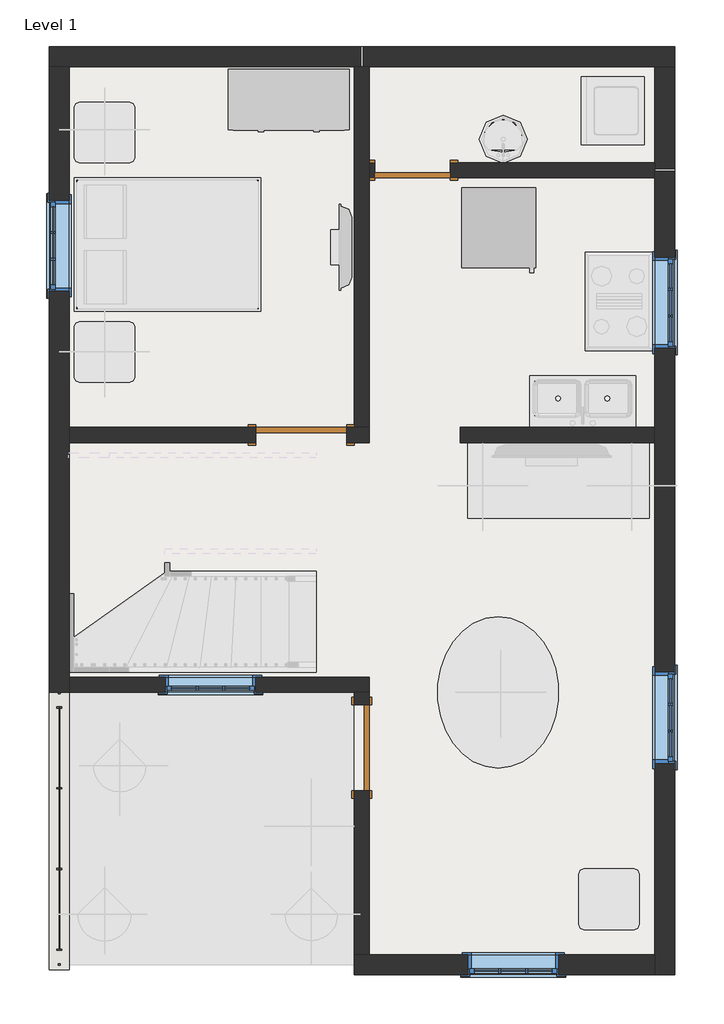
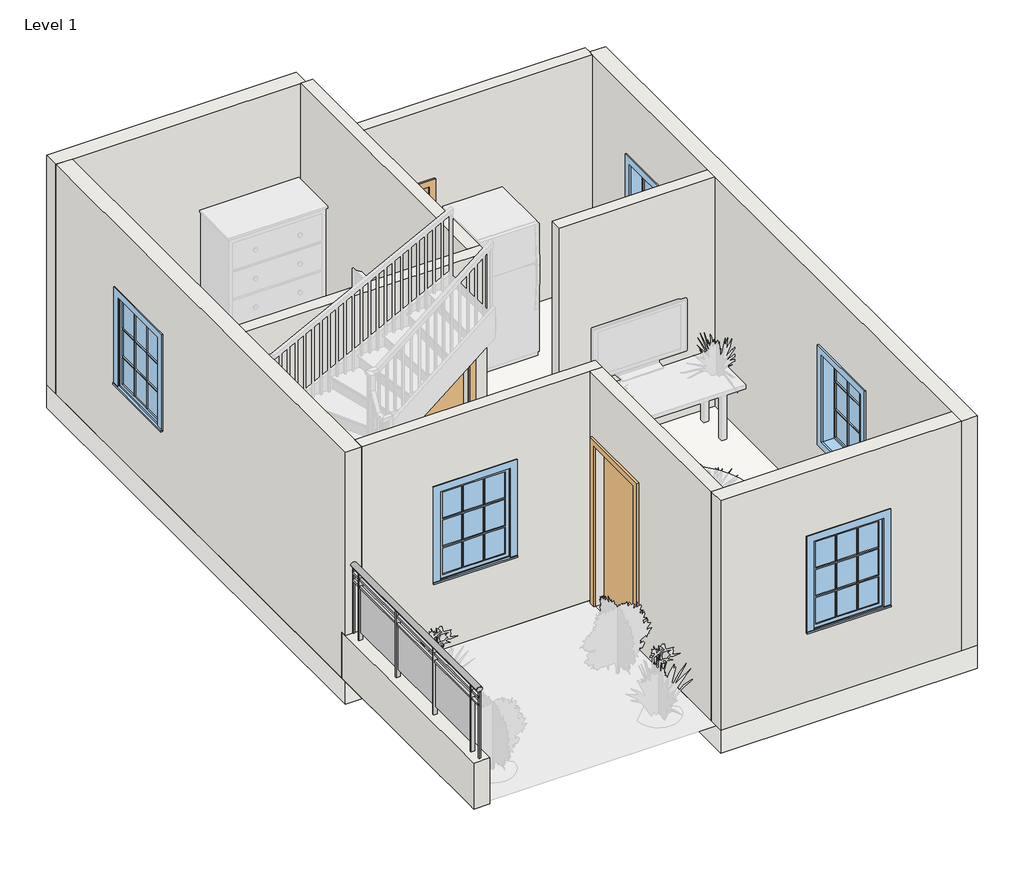
# One storey, part 1 of 3: 13 walls, 5 windows, 3 doors, 1 railing, 1 slab.
"""IFC4 building model written with IfcOpenShell, lengths in millimetres."""

from ifc_helpers import new_model, si_unit, point, frame, origin, origin_with_axes, place, context, project, spatial, polyline, ellipse_curve, trimmed, outline, extrude, faceted_brep, transform, mapped, element, save
from ifc_brep_helpers import plane_surface, extruded_surface, advanced_brep
from components import door_059fdd7e, door_b6e9fca3, door_16372e1c, window_29c06734, window_5c190c7e

model = new_model("IFC4")

# Units and contexts
model_context = context("Model", 3, world=origin())
ifc_project = project(units=[si_unit("LENGTHUNIT", "METRE", prefix="MILLI")], contexts=[model_context])

# Site, building, storey
site = spatial("IfcSite", under=ifc_project)
building = spatial("IfcBuilding", under=site)
storey = spatial("IfcBuildingStorey", under=building, Name="Level 1", Elevation=0.0)

# Doors
placement = place(None, origin())
door_shape = door_059fdd7e(model_context)
element("IfcDoor", 1, ObjectType="Single-Flush : 30\" x 80\"", at=placement, inside=storey, context=model_context, shape_type="MappedRepresentation", body=[
    mapped(door_shape, transform((-13127.2170266, 11870.4465295, 0.0), x_axis=(-1.0, 0.0, 0.0), y_axis=(0.0, -1.0, 0.0), z_axis=(0.0, 0.0, 1.0))),
])
door_2_shape = door_b6e9fca3(model_context)
element("IfcDoor", 2, ObjectType="Single-Flush : 34\" x 84\"", at=placement, inside=storey, context=model_context, shape_type="MappedRepresentation", body=[
    mapped(door_2_shape, transform((-13635.2170266, 6053.8465295, 0.0), x_axis=(0.0, -1.0, 0.0), y_axis=(1.0, 0.0, 0.0), z_axis=(0.0, 0.0, 1.0))),
])
door_3_shape = door_16372e1c(model_context)
element("IfcDoor", 3, ObjectType="Single-Flush : 36\" x 84\"", at=placement, inside=storey, context=model_context, shape_type="MappedRepresentation", body=[
    mapped(door_3_shape, transform((-14244.8170266, 9203.4465295, 0.0), x_axis=(1.0, 0.0, 0.0), y_axis=(0.0, 1.0, 0.0), z_axis=(0.0, 0.0, 1.0))),
])

# Railing
element("IfcRailing", 4, ObjectType="Glass Panel - Bottom Fill", at=placement, inside=storey, context=model_context, shape_type="SolidModel", body=[
    advanced_brep(
    [(-16645.1170266, 6612.6465295, 1524.0), (-16721.3170266, 6612.6465295, 1524.0), (-16645.1170266, 3869.4465295, 1524.0), (-16721.3170266, 3869.4465295, 1524.0)],
    [
        (0, 1, ellipse_curve(frame((-16683.2170266, 6612.6465295, 1524.0), z_axis=(0.0, 1.0, 0.0), x_axis=(-1.0, 0.0, 0.0)), 38.1, 28.575)),
        (1, 0, ellipse_curve(frame((-16683.2170266, 6612.6465295, 1524.0), z_axis=(0.0, 1.0, 0.0), x_axis=(-1.0, 0.0, 0.0)), 38.1, 28.575)),
        (2, 3, ellipse_curve(frame((-16683.2170266, 3869.4465295, 1524.0), z_axis=(0.0, -1.0, 0.0), x_axis=(-1.0, 0.0, 0.0)), 38.1, 28.575)),
        (3, 2, ellipse_curve(frame((-16683.2170266, 3869.4465295, 1524.0), z_axis=(0.0, -1.0, 0.0), x_axis=(-1.0, 0.0, 0.0)), 38.1, 28.575)),
        (0, 2),
        (3, 1),
    ],
    [
        plane_surface(frame((-16683.2170266, 6612.6465295, 1524.0), z_axis=(0.0, 1.0, 0.0), x_axis=(0.0, 0.0, -1.0))),
        plane_surface(frame((-16683.2170266, 3869.4465295, 1524.0), z_axis=(0.0, -1.0, 0.0), x_axis=(0.0, 0.0, -1.0))),
        extruded_surface(trimmed(ellipse_curve(frame((-16683.2170266, 3869.4465295, 1524.0), z_axis=(0.0, 1.0, 0.0), x_axis=(-1.0, 0.0, 0.0)), 38.1, 28.575), [point((-16645.1170266, 3869.4465295, 1524.0))], [point((-16721.3170266, 3869.4465295, 1524.0))], True, "CARTESIAN"), (0.0, 2743.2, 0.0), 2743.2),
        extruded_surface(trimmed(ellipse_curve(frame((-16683.2170266, 3869.4465295, 1524.0), z_axis=(0.0, 1.0, 0.0), x_axis=(-1.0, 0.0, 0.0)), 38.1, 28.575), [point((-16721.3170266, 3869.4465295, 1524.0))], [point((-16645.1170266, 3869.4465295, 1524.0))], True, "CARTESIAN"), (0.0, 2743.2, 0.0), 2743.2),
    ],
    [
        (0, [[1, 2]]),
        (1, [[3, 4]]),
        (2, [[-1, 5, -4, 6]]),
        (3, [[-2, -6, -3, -5]]),
    ],
),
    extrude(outline(polyline([(-16695.9170266, 6612.6465295), (-16670.5170266, 6612.6465295), (-16670.5170266, 3869.4465295), (-16695.9170266, 3869.4465295), (-16695.9170266, 6612.6465295)])), frame((0.0, 0.0, 1409.7), z_axis=(0.0, 0.0, 1.0), x_axis=(1.0, 0.0, 0.0)), (0.0, 0.0, 1.0), 25.4),
    extrude(outline(polyline([(-16695.9170266, 6612.6465295), (-16670.5170266, 6612.6465295), (-16670.5170266, 3869.4465295), (-16695.9170266, 3869.4465295), (-16695.9170266, 6612.6465295)])), frame((0.0, 0.0, 1308.1), z_axis=(0.0, 0.0, 1.0), x_axis=(1.0, 0.0, 0.0)), (0.0, 0.0, 1.0), 25.4),
    extrude(outline(polyline([(-16708.6170266, 4028.1965295), (-16657.8170266, 4028.1965295), (-16657.8170266, 4015.4965295), (-16708.6170266, 4015.4965295), (-16708.6170266, 4028.1965295)])), frame((0.0, 0.0, 609.6), z_axis=(0.0, 0.0, 1.0), x_axis=(1.0, 0.0, 0.0)), (0.0, 0.0, 1.0), 885.6788223),
    extrude(outline(polyline([(-16676.6818696, 4834.6465295), (-16676.6818696, 4021.8465295), (-16683.0318696, 4021.8465295), (-16683.0318696, 4834.6465295), (-16676.6818696, 4834.6465295)])), frame((0.0, 0.0, 711.2), z_axis=(0.0, 0.0, 1.0), x_axis=(1.0, 0.0, 0.0)), (0.0, 0.0, 1.0), 596.9),
    extrude(outline(polyline([(-16708.6170266, 4840.9965295), (-16657.8170266, 4840.9965295), (-16657.8170266, 4828.2965295), (-16708.6170266, 4828.2965295), (-16708.6170266, 4840.9965295)])), frame((0.0, 0.0, 609.6), z_axis=(0.0, 0.0, 1.0), x_axis=(1.0, 0.0, 0.0)), (0.0, 0.0, 1.0), 885.6788223),
    extrude(outline(polyline([(-16676.6818696, 5647.4465295), (-16676.6818696, 4834.6465295), (-16683.0318696, 4834.6465295), (-16683.0318696, 5647.4465295), (-16676.6818696, 5647.4465295)])), frame((0.0, 0.0, 711.2), z_axis=(0.0, 0.0, 1.0), x_axis=(1.0, 0.0, 0.0)), (0.0, 0.0, 1.0), 596.9),
    extrude(outline(polyline([(-16708.6170266, 5653.7965295), (-16657.8170266, 5653.7965295), (-16657.8170266, 5641.0965295), (-16708.6170266, 5641.0965295), (-16708.6170266, 5653.7965295)])), frame((0.0, 0.0, 609.6), z_axis=(0.0, 0.0, 1.0), x_axis=(1.0, 0.0, 0.0)), (0.0, 0.0, 1.0), 885.6788223),
    extrude(outline(polyline([(-16676.6818696, 6460.2465295), (-16676.6818696, 5647.4465295), (-16683.0318696, 5647.4465295), (-16683.0318696, 6460.2465295), (-16676.6818696, 6460.2465295)])), frame((0.0, 0.0, 711.2), z_axis=(0.0, 0.0, 1.0), x_axis=(1.0, 0.0, 0.0)), (0.0, 0.0, 1.0), 596.9),
    extrude(outline(polyline([(-16708.6170266, 6466.5965295), (-16657.8170266, 6466.5965295), (-16657.8170266, 6453.8965295), (-16708.6170266, 6453.8965295), (-16708.6170266, 6466.5965295)])), frame((0.0, 0.0, 609.6), z_axis=(0.0, 0.0, 1.0), x_axis=(1.0, 0.0, 0.0)), (0.0, 0.0, 1.0), 885.6788223),
    extrude(outline(polyline([(-16692.7420266, 3882.1465295), (-16673.6920266, 3882.1465295), (-16673.6920266, 3863.0965295), (-16692.7420266, 3863.0965295), (-16692.7420266, 3882.1465295)])), frame((0.0, 0.0, 609.6), z_axis=(0.0, 0.0, 1.0), x_axis=(1.0, 0.0, 0.0)), (0.0, 0.0, 1.0), 885.6788223),
    extrude(outline(polyline([(-16692.7420266, 6618.9965295), (-16673.6920266, 6618.9965295), (-16673.6920266, 6599.9465295), (-16692.7420266, 6599.9465295), (-16692.7420266, 6618.9965295)])), frame((0.0, 0.0, 609.6), z_axis=(0.0, 0.0, 1.0), x_axis=(1.0, 0.0, 0.0)), (0.0, 0.0, 1.0), 885.6788223),
])

# Slab
element("IfcSlab", 5, ObjectType="Generic - 12\"", at=placement, inside=storey, context=model_context, shape_type="SweptSolid", body=[
    extrude(outline(polyline([(-10485.6170266, 13115.0465295), (-10485.6170266, 3767.8465295), (-13711.4170266, 3767.8465295), (-13711.4170266, 6612.6465295), (-16784.8170266, 6612.6465295), (-16784.8170266, 13115.0465295), (-10485.6170266, 13115.0465295)])), frame((0.0, 0.0, -304.8), z_axis=(0.0, 0.0, 1.0), x_axis=(1.0, 0.0, 0.0)), (0.0, 0.0, 1.0), 304.8),
])

# Walls
element("IfcWall", 6, ObjectType="Generic - 8\"", at=placement, inside=storey, context=model_context, shape_type="Brep", body=[
    faceted_brep([(-13711.4170266, 12911.8465295, 0.0), (-13711.4170266, 9279.6465295, 0.0), (-13711.4170266, 9279.6465295, 3048.0), (-13711.4170266, 12911.8465295, 3048.0), (-13559.0170266, 12911.8465295, 0.0), (-13559.0170266, 12911.8465295, 3048.0), (-13559.0170266, 11946.6465295, 3048.0), (-13559.0170266, 11794.2465295, 3048.0), (-13559.0170266, 9279.6465295, 3048.0), (-13559.0170266, 9279.6465295, 0.0), (-13559.0170266, 11794.2465295, 0.0), (-13559.0170266, 11946.6465295, 0.0), (-13622.5170266, 12911.8465295, 0.0)], [[[0, 1, 2, 3]], [[4, 5, 6, 7, 8, 9, 10, 11]], [[1, 0, 12, 4, 11, 10, 9]], [[3, 2, 8, 7, 6, 5]], [[0, 3, 5, 4, 12]], [[2, 1, 9, 8]]]),
])
element("IfcWall", 7, ObjectType="Generic - 8\"", at=placement, inside=storey, context=model_context, shape_type="SweptSolid", body=[
    extrude(outline(polyline([(-12644.6170266, 9279.6465295), (-10688.8170266, 9279.6465295), (-10688.8170266, 9127.2465295), (-12644.6170266, 9127.2465295), (-12644.6170266, 9279.6465295)])), origin_with_axes(), (0.0, 0.0, 1.0), 3048.0),
])
element("IfcWall", 8, ObjectType="Generic - 8\"", at=placement, inside=storey, context=model_context, shape_type="Brep", body=[
    faceted_brep([(-13559.0170266, 11794.2465295, 0.0), (-13508.2170266, 11794.2465295, 0.0), (-13508.2170266, 11794.2465295, 2032.0), (-12746.2170266, 11794.2465295, 2032.0), (-12746.2170266, 11794.2465295, 0.0), (-10688.8170266, 11794.2465295, 0.0), (-10688.8170266, 11794.2465295, 3048.0), (-13559.0170266, 11794.2465295, 3048.0), (-13508.2170266, 11946.6465295, 2032.0), (-13508.2170266, 11946.6465295, 0.0), (-13559.0170266, 11946.6465295, 0.0), (-13559.0170266, 11946.6465295, 3048.0), (-10688.8170266, 11946.6465295, 3048.0), (-10688.8170266, 11946.6465295, 0.0), (-12746.2170266, 11946.6465295, 0.0), (-12746.2170266, 11946.6465295, 2032.0), (-10688.8170266, 11857.7465295, 0.0), (-10688.8170266, 11857.7465295, 3048.0)], [[[0, 1, 2, 3, 4, 5, 6, 7]], [[8, 9, 10, 11, 12, 13, 14, 15]], [[14, 13, 16, 5, 4]], [[10, 9, 1, 0]], [[7, 6, 17, 12, 11]], [[6, 5, 16, 13, 12, 17]], [[0, 7, 11, 10]], [[2, 1, 9, 8]], [[3, 2, 8, 15]], [[4, 3, 15, 14]]]),
])
element("IfcWall", 9, ObjectType="Generic - 8\"", at=placement, inside=storey, context=model_context, shape_type="Brep", body=[
    faceted_brep([(-16581.6170266, 6612.6465295, 3048.0), (-16581.6170266, 6612.6465295, 609.6), (-16581.6170266, 6612.6465295, 0.0), (-13711.4170266, 6612.6465295, 0.0), (-13559.0170266, 6612.6465295, 0.0), (-13559.0170266, 6612.6465295, 3048.0), (-13711.4170266, 6612.6465295, 3048.0), (-15616.4170266, 6612.6465295, 2133.6), (-14702.0170266, 6612.6465295, 2133.6), (-14702.0170266, 6612.6465295, 914.4), (-15616.4170266, 6612.6465295, 914.4), (-16581.6170266, 6765.0465295, 0.0), (-16581.6170266, 6765.0465295, 3048.0), (-13559.0170266, 6765.0465295, 3048.0), (-13559.0170266, 6765.0465295, 0.0), (-15616.4170266, 6765.0465295, 2133.6), (-15616.4170266, 6765.0465295, 914.4), (-14702.0170266, 6765.0465295, 914.4), (-14702.0170266, 6765.0465295, 2133.6), (-16581.6170266, 6688.8465295, 0.0)], [[[0, 1, 2, 3, 4, 5, 6], [7, 8, 9, 10]], [[11, 12, 13, 14], [15, 16, 17, 18]], [[4, 3, 2, 19, 11, 14]], [[0, 6, 5, 13, 12]], [[5, 4, 14, 13]], [[0, 12, 11, 19, 2, 1]], [[16, 15, 7, 10]], [[17, 16, 10, 9]], [[18, 17, 9, 8]], [[15, 18, 8, 7]]]),
])
element("IfcWall", 10, ObjectType="Generic - 8\"", at=placement, inside=storey, context=model_context, shape_type="SweptSolid", body=[
    extrude(outline(polyline([(5622.0465295, 2133.6), (5622.0465295, 0.0), (3971.0465295, 0.0), (3971.0465295, 3048.0), (6612.6465295, 3048.0), (6612.6465295, 0.0), (6485.6465295, 0.0), (6485.6465295, 2133.6), (5622.0465295, 2133.6)])), frame((-13711.4170266, 0.0, 0.0), z_axis=(1.0, 0.0, 0.0), x_axis=(0.0, 1.0, 0.0)), (0.0, 0.0, 1.0), 152.4),
])
element("IfcWall", 11, ObjectType="Generic - 8\"", at=placement, inside=storey, context=model_context, shape_type="Brep", body=[
    faceted_brep([(-13559.0170266, 9279.6465295, 0.0), (-13711.4170266, 9279.6465295, 0.0), (-13787.6170266, 9279.6465295, 0.0), (-13787.6170266, 9279.6465295, 2133.6), (-14702.0170266, 9279.6465295, 2133.6), (-14702.0170266, 9279.6465295, 0.0), (-16581.6170266, 9279.6465295, 0.0), (-16581.6170266, 9279.6465295, 3048.0), (-13711.4170266, 9279.6465295, 3048.0), (-13559.0170266, 9279.6465295, 3048.0), (-13787.6170266, 9127.2465295, 2133.6), (-13787.6170266, 9127.2465295, 0.0), (-13559.0170266, 9127.2465295, 0.0), (-13559.0170266, 9127.2465295, 3048.0), (-16581.6170266, 9127.2465295, 3048.0), (-16581.6170266, 9127.2465295, 0.0), (-14702.0170266, 9127.2465295, 0.0), (-14702.0170266, 9127.2465295, 2133.6)], [[[0, 1, 2, 3, 4, 5, 6, 7, 8, 9]], [[10, 11, 12, 13, 14, 15, 16, 17]], [[16, 15, 6, 5]], [[12, 11, 2, 1, 0]], [[9, 8, 7, 14, 13]], [[7, 6, 15, 14]], [[5, 4, 17, 16]], [[4, 3, 10, 17]], [[3, 2, 11, 10]], [[0, 9, 13, 12]]]),
])
element("IfcWall", 12, ObjectType="Generic - 8\" 2", at=placement, inside=storey, context=model_context, shape_type="Brep", body=[
    faceted_brep([(-16784.8170266, 12911.8465295, 0.0), (-16581.6170266, 12911.8465295, 0.0), (-13647.9170266, 12911.8465295, 0.0), (-13647.9170266, 12911.8465295, 3048.0), (-16581.6170266, 12911.8465295, 3048.0), (-16784.8170266, 12911.8465295, 3048.0), (-16784.8170266, 13115.0465295, 0.0), (-16784.8170266, 13115.0465295, 3048.0), (-13647.9170266, 13115.0465295, 3048.0), (-13647.9170266, 13115.0465295, 0.0)], [[[0, 1, 2, 3, 4, 5]], [[6, 7, 8, 9]], [[2, 1, 0, 6, 9]], [[3, 2, 9, 8]], [[5, 4, 3, 8, 7]], [[0, 5, 7, 6]]]),
])
element("IfcWall", 13, ObjectType="Generic - 8\" 2", at=placement, inside=storey, context=model_context, shape_type="SweptSolid", body=[
    extrude(outline(polyline([(-10688.8170266, 11883.1465295), (-10688.8170266, 12911.8465295), (-10485.6170266, 12911.8465295), (-10485.6170266, 11883.1465295), (-10688.8170266, 11883.1465295)])), origin_with_axes(), (0.0, 0.0, 1.0), 1524.0),
])
element("IfcWall", 14, ObjectType="Generic - 8\" 2", at=placement, inside=storey, context=model_context, shape_type="Brep", body=[
    faceted_brep([(-10688.8170266, 3971.0465295, 0.0), (-13559.0170266, 3971.0465295, 0.0), (-13711.4170266, 3971.0465295, 0.0), (-13711.4170266, 3971.0465295, 3048.0), (-13559.0170266, 3971.0465295, 3048.0), (-10688.8170266, 3971.0465295, 3048.0), (-12568.4170266, 3971.0465295, 2133.6), (-12568.4170266, 3971.0465295, 914.4), (-11654.0170266, 3971.0465295, 914.4), (-11654.0170266, 3971.0465295, 2133.6), (-10688.8170266, 3767.8465295, 0.0), (-10688.8170266, 3767.8465295, 3048.0), (-13711.4170266, 3767.8465295, 3048.0), (-13711.4170266, 3767.8465295, 0.0), (-12568.4170266, 3767.8465295, 2133.6), (-11654.0170266, 3767.8465295, 2133.6), (-11654.0170266, 3767.8465295, 914.4), (-12568.4170266, 3767.8465295, 914.4)], [[[0, 1, 2, 3, 4, 5], [6, 7, 8, 9]], [[10, 11, 12, 13], [14, 15, 16, 17]], [[2, 1, 0, 10, 13]], [[5, 4, 3, 12, 11]], [[0, 5, 11, 10]], [[3, 2, 13, 12]], [[7, 6, 14, 17]], [[8, 7, 17, 16]], [[9, 8, 16, 15]], [[6, 9, 15, 14]]]),
])
element("IfcWall", 15, ObjectType="Generic - 8\" 2", at=placement, inside=storey, context=model_context, shape_type="Brep", body=[
    faceted_brep([(-13622.5170266, 12911.8465295, 0.0), (-13559.0170266, 12911.8465295, 0.0), (-10688.8170266, 12911.8465295, 0.0), (-10485.6170266, 12911.8465295, 0.0), (-10485.6170266, 12911.8465295, 1524.0), (-10688.8170266, 12911.8465295, 1524.0), (-13622.5170266, 12911.8465295, 1524.0), (-13622.5170266, 13115.0465295, 0.0), (-13622.5170266, 13115.0465295, 1524.0), (-10485.6170266, 13115.0465295, 1524.0), (-10485.6170266, 13115.0465295, 0.0)], [[[0, 1, 2, 3, 4, 5, 6]], [[7, 8, 9, 10]], [[3, 2, 1, 0, 7, 10]], [[6, 5, 4, 9, 8]], [[0, 6, 8, 7]], [[4, 3, 10, 9]]]),
])
element("IfcWall", 16, ObjectType="Generic - 8\" 2", at=placement, inside=storey, context=model_context, shape_type="Brep", body=[
    faceted_brep([(-10688.8170266, 11857.7465295, 0.0), (-10688.8170266, 11794.2465295, 0.0), (-10688.8170266, 9279.6465295, 0.0), (-10688.8170266, 9127.2465295, 0.0), (-10688.8170266, 3971.0465295, 0.0), (-10688.8170266, 3767.8465295, 0.0), (-10688.8170266, 3767.8465295, 3048.0), (-10688.8170266, 3971.0465295, 3048.0), (-10688.8170266, 9127.2465295, 3048.0), (-10688.8170266, 9279.6465295, 3048.0), (-10688.8170266, 11794.2465295, 3048.0), (-10688.8170266, 11857.7465295, 3048.0), (-10688.8170266, 10079.7465295, 2133.6), (-10688.8170266, 10079.7465295, 914.4), (-10688.8170266, 10994.1465295, 914.4), (-10688.8170266, 10994.1465295, 2133.6), (-10688.8170266, 5901.4465295, 2133.6), (-10688.8170266, 5901.4465295, 914.4), (-10688.8170266, 6815.8465295, 914.4), (-10688.8170266, 6815.8465295, 2133.6), (-10485.6170266, 11857.7465295, 0.0), (-10485.6170266, 11857.7465295, 3048.0), (-10485.6170266, 3767.8465295, 3048.0), (-10485.6170266, 3767.8465295, 0.0), (-10485.6170266, 10079.7465295, 2133.6), (-10485.6170266, 10994.1465295, 2133.6), (-10485.6170266, 10994.1465295, 914.4), (-10485.6170266, 10079.7465295, 914.4), (-10485.6170266, 5901.4465295, 2133.6), (-10485.6170266, 6815.8465295, 2133.6), (-10485.6170266, 6815.8465295, 914.4), (-10485.6170266, 5901.4465295, 914.4)], [[[0, 1, 2, 3, 4, 5, 6, 7, 8, 9, 10, 11], [12, 13, 14, 15], [16, 17, 18, 19]], [[20, 21, 22, 23], [24, 25, 26, 27], [28, 29, 30, 31]], [[5, 4, 3, 2, 1, 0, 20, 23]], [[11, 10, 9, 8, 7, 6, 22, 21]], [[0, 11, 21, 20]], [[6, 5, 23, 22]], [[13, 12, 24, 27]], [[14, 13, 27, 26]], [[15, 14, 26, 25]], [[12, 15, 25, 24]], [[17, 16, 28, 31]], [[18, 17, 31, 30]], [[19, 18, 30, 29]], [[16, 19, 29, 28]]]),
])
element("IfcWall", 17, ObjectType="Generic - 8\" 2", at=placement, inside=storey, context=model_context, shape_type="Brep", body=[
    faceted_brep([(-16581.6170266, 6688.8465295, 0.0), (-16581.6170266, 6765.0465295, 0.0), (-16581.6170266, 9127.2465295, 0.0), (-16581.6170266, 9279.6465295, 0.0), (-16581.6170266, 12911.8465295, 0.0), (-16581.6170266, 12911.8465295, 3048.0), (-16581.6170266, 9279.6465295, 3048.0), (-16581.6170266, 9127.2465295, 3048.0), (-16581.6170266, 6765.0465295, 3048.0), (-16581.6170266, 6612.6465295, 3048.0), (-16581.6170266, 6612.6465295, 609.6), (-16581.6170266, 6688.8465295, 609.6), (-16581.6170266, 11565.6465295, 2133.6), (-16581.6170266, 11565.6465295, 914.4), (-16581.6170266, 10651.2465295, 914.4), (-16581.6170266, 10651.2465295, 2133.6), (-16784.8170266, 6688.8465295, 0.0), (-16784.8170266, 6688.8465295, 609.6), (-16784.8170266, 6612.6465295, 609.6), (-16784.8170266, 6612.6465295, 3048.0), (-16784.8170266, 12911.8465295, 3048.0), (-16784.8170266, 12911.8465295, 0.0), (-16784.8170266, 11565.6465295, 2133.6), (-16784.8170266, 10651.2465295, 2133.6), (-16784.8170266, 10651.2465295, 914.4), (-16784.8170266, 11565.6465295, 914.4)], [[[0, 1, 2, 3, 4, 5, 6, 7, 8, 9, 10, 11], [12, 13, 14, 15]], [[16, 17, 18, 19, 20, 21], [22, 23, 24, 25]], [[4, 3, 2, 1, 0, 16, 21]], [[9, 8, 7, 6, 5, 20, 19]], [[5, 4, 21, 20]], [[12, 15, 23, 22]], [[15, 14, 24, 23]], [[14, 13, 25, 24]], [[13, 12, 22, 25]], [[0, 11, 17, 16]], [[10, 18, 17, 11]], [[10, 9, 19, 18]]]),
])
element("IfcWall", 18, ObjectType="Generic - 8\" 3", at=placement, inside=storey, context=model_context, shape_type="Brep", body=[
    faceted_brep([(-16581.6170266, 3818.6465295, 0.0), (-16581.6170266, 6612.6465295, 0.0), (-16581.6170266, 6688.8465295, 0.0), (-16581.6170266, 6688.8465295, 609.6), (-16581.6170266, 3818.6465295, 609.6), (-16784.8170266, 3818.6465295, 0.0), (-16784.8170266, 3818.6465295, 609.6), (-16784.8170266, 6688.8465295, 609.6), (-16784.8170266, 6688.8465295, 0.0)], [[[0, 1, 2, 3, 4]], [[5, 6, 7, 8]], [[2, 1, 0, 5, 8]], [[3, 2, 8, 7]], [[4, 3, 7, 6]], [[0, 4, 6, 5]]]),
])

# Windows
window_shape = window_29c06734(model_context)
element("IfcWindow", 19, ObjectType="Casement 3x3 with Trim : 36\" x 48\"", at=placement, inside=storey, context=model_context, shape_type="MappedRepresentation", body=[
    mapped(window_shape, transform((-16683.2170266, 11108.4465295, 0.0), x_axis=(0.0, 1.0, 0.0), y_axis=(-1.0, 0.0, 0.0), z_axis=(0.0, 0.0, 1.0))),
])
element("IfcWindow", 20, ObjectType="Casement 3x3 with Trim : 36\" x 48\"", at=placement, inside=storey, context=model_context, shape_type="MappedRepresentation", body=[
    mapped(window_shape, transform((-10587.2170266, 10536.9465295, 0.0), x_axis=(0.0, -1.0, 0.0), y_axis=(1.0, 0.0, 0.0), z_axis=(0.0, 0.0, 1.0))),
])
element("IfcWindow", 21, ObjectType="Casement 3x3 with Trim : 36\" x 48\"", at=placement, inside=storey, context=model_context, shape_type="MappedRepresentation", body=[
    mapped(window_shape, transform((-12111.2170266, 3869.4465295, 0.0), x_axis=(-1.0, 0.0, 0.0), y_axis=(0.0, -1.0, 0.0), z_axis=(0.0, 0.0, 1.0))),
])
element("IfcWindow", 22, ObjectType="Casement 3x3 with Trim : 36\" x 48\"", at=placement, inside=storey, context=model_context, shape_type="MappedRepresentation", body=[
    mapped(window_shape, transform((-10587.2170266, 6358.6465295, 0.0), x_axis=(0.0, -1.0, 0.0), y_axis=(1.0, 0.0, 0.0), z_axis=(0.0, 0.0, 1.0))),
])
window_2_shape = window_5c190c7e(model_context)
element("IfcWindow", 23, ObjectType="Casement 3x3 with Trim : 36\" x 48\"", at=placement, inside=storey, context=model_context, shape_type="MappedRepresentation", body=[
    mapped(window_2_shape, transform((-15159.2170266, 6688.8465295, 0.0), x_axis=(-1.0, 0.0, 0.0), y_axis=(0.0, -1.0, 0.0), z_axis=(0.0, 0.0, 1.0))),
])

save(model, "model.ifc")

# Revit data of these elements
# Type "Single-Flush : 30\" x 80\""
#   Type Mark = "5"
#   Construction Type Id = "MDOOR"
#   Assembly Code = "C1020"
#   Analytic Construction = "Metal"
#   Thickness = 0' - 2"
#   Heat Transfer Coefficient (U) = 0.651978 BTU/(h·ft²·°F)
#   Height = 6' - 8"
#   Trim Projection Ext = 0' - 1"
#   Trim Projection Int = 0' - 1"
#   Trim Width = 0' - 3"
#   Width = 2' - 6"
#   Define Thermal Properties by = 1
#   Door Material = Door - Panel
#   Frame Material = Door - Frame
#   Visual Light Transmittance = 0
#   Solar Heat Gain Coefficient = 0
#   Function = (empty or 0)
#   Wall Closure = (empty or 0)
# Type "Single-Flush : 34\" x 84\""
#   Type Mark = "2"
#   Construction Type Id = "MDOOR"
#   Assembly Code = "C1020"
#   Analytic Construction = "Metal"
#   Thickness = 0' - 2"
#   Heat Transfer Coefficient (U) = 0.651978 BTU/(h·ft²·°F)
#   Height = 7' - 0"
#   Trim Projection Ext = 0' - 1"
#   Trim Projection Int = 0' - 1"
#   Trim Width = 0' - 3"
#   Width = 2' - 10"
#   Define Thermal Properties by = 1
#   Door Material = Door - Panel
#   Frame Material = Door - Frame
#   Visual Light Transmittance = 0
#   Solar Heat Gain Coefficient = 0
#   Function = (empty or 0)
#   Wall Closure = (empty or 0)
# Type "Single-Flush : 36\" x 84\""
#   Type Mark = "1"
#   Construction Type Id = "MDOOR"
#   Assembly Code = "C1020"
#   Analytic Construction = "Metal"
#   Thickness = 0' - 2"
#   Heat Transfer Coefficient (U) = 0.651978 BTU/(h·ft²·°F)
#   Height = 7' - 0"
#   Trim Projection Ext = 0' - 1"
#   Trim Projection Int = 0' - 1"
#   Trim Width = 0' - 3"
#   Width = 3' - 0"
#   Define Thermal Properties by = 1
#   Door Material = Door - Panel
#   Frame Material = Door - Frame
#   Visual Light Transmittance = 0
#   Solar Heat Gain Coefficient = 0
#   Function = (empty or 0)
#   Wall Closure = (empty or 0)
# Type "Glass Panel - Bottom Fill"
#   Assembly Code = "C2010400"
#   built-in parameter 1008612 = 0.0416667 (stored number, unit not read)
#   built-in parameter 1008611 = 0.0416667 (stored number, unit not read)
#   built-in parameter 1008609 = 0.333333 (stored number, unit not read)
#   built-in parameter 1008604 = 0.166667 (stored number, unit not read)
#   built-in parameter 1008603 = 0.166667 (stored number, unit not read)
#   Railing Height = 3' - 0"
#   built-in parameter 1008630 = 2
#   built-in parameter 1008610 = 2
#   built-in parameter 1008618 = Baluster - Square : 3/4"
# Type "Generic - 12\""
#   Assembly Code = "B1010"
#   Function = 0
#   Layers, outside or top first: 1' - 0" "Brick, Common" (function 1)
# Type "Generic - 8\""
#   Assembly Code = "B2010"
#   Layers, outside or top first: 0' - 6" "Brick, Common" (function 1)
# Type "Generic - 8\" 2"
#   Assembly Code = "B2010"
#   Layers, outside or top first: 0' - 8" "Brick, Common" (function 1)
# Type "Generic - 8\" 3"
#   Assembly Code = "B2010"
#   Layers, outside or top first: 0' - 8" "Birch" (function 1)
# Type "Casement 3x3 with Trim : 36\" x 48\""
#   Type Mark = "10"
#   Construction Type Id = "GSP4R"
#   Assembly Code = "B2020100"
#   Analytic Construction = "1/8 in Pilkington single glazing"
#   Visual Light Transmittance = 0.9
#   Solar Heat Gain Coefficient = 0.78
#   Heat Transfer Coefficient (U) = 0.6496 BTU/(h·ft²·°F)
#   Height = 4' - 0"
#   Default Sill Height = 3' - 0"
#   Trim Projection - Ext. = 0' - 0 1/2"
#   Trim Projection - Int. = 0' - 0 3/4"
#   Trim Width - Exterior = 0' - 3 1/2"
#   Trim Width - Interior = 0' - 3 1/2"
#   Width = 3' - 0"
#   Window Inset = 0' - 0 3/4"
#   Define Thermal Properties by = 1
#   Glass Pane Material = Glass
#   Sash Material = Sash
#   Trim Exterior Material = Trim
#   Trim Interior Material = Trim
#   Wall Closure = (empty or 0)
# Element 1 (IfcDoor, "Single-Flush : 30\" x 80\"")
#   Phase Created = New Construction
#   Materials on its faces: "Door - Frame", "Door - Panel"
# Element 2 (IfcDoor, "Single-Flush : 34\" x 84\"")
#   Phase Created = New Construction
#   Materials on its faces: "Door - Frame", "Door - Panel"
# Element 3 (IfcDoor, "Single-Flush : 36\" x 84\"")
#   Phase Created = New Construction
#   Materials on its faces: "Door - Frame", "Door - Panel"
# Element 4 (IfcRailing, "Glass Panel - Bottom Fill")
#   built-in parameter 1008621 = 2 (stored number, unit not read)
#   Phase Created = New Construction
#   Materials on its faces: "Glass"
# Element 5 (IfcSlab, "Generic - 12\"")
#   Height Offset From Level = 0' - 0"
#   Phase Created = New Construction
#   Materials on its faces: "Brick, Common"
# Elements 6, 7, 8, 9, 10, 11 (IfcWall, "Generic - 8\"")
#   Top Offset = 0' - 0"
#   Base Offset = 0' - 0"
#   Unconnected Height = 10' - 0"
#   wall height = 10' - 0"
#   Phase Created = New Construction
#   Base Constraint = Level 1
#   Materials on its faces: "Brick, Common"
# Elements 12, 14, 16, 17 (IfcWall, "Generic - 8\" 2")
#   Top Offset = 0' - 0"
#   Base Offset = 0' - 0"
#   Unconnected Height = 10' - 0"
#   wall height = 10' - 0"
#   Phase Created = New Construction
#   Base Constraint = Level 1
#   Materials on its faces: "Brick, Common"
# Elements 13, 15 (IfcWall, "Generic - 8\" 2")
#   Top Offset = 0' - 0"
#   Base Offset = 0' - 0"
#   Unconnected Height = 5' - 0"
#   wall height = 5' - 0"
#   Phase Created = New Construction
#   Base Constraint = Level 1
#   Materials on its faces: "Brick, Common"
# Element 18 (IfcWall, "Generic - 8\" 3")
#   Top Offset = 0' - 0"
#   Base Offset = 0' - 0"
#   Unconnected Height = 2' - 0"
#   wall height = 2' - 0"
#   Phase Created = New Construction
#   Base Constraint = Level 1
#   Materials on its faces: "Birch"
# Element 19 (IfcWindow, "Casement 3x3 with Trim : 36\" x 48\"")
#   Mark = "1"
#   Phase Created = New Construction
#   Materials on its faces: "Sash", "Glass", "Trim"
# Element 20 (IfcWindow, "Casement 3x3 with Trim : 36\" x 48\"")
#   Mark = "2"
#   Phase Created = New Construction
#   Materials on its faces: "Sash", "Glass", "Trim"
# Element 21 (IfcWindow, "Casement 3x3 with Trim : 36\" x 48\"")
#   Mark = "4"
#   Phase Created = New Construction
#   Materials on its faces: "Sash", "Glass", "Trim"
# Element 22 (IfcWindow, "Casement 3x3 with Trim : 36\" x 48\"")
#   Mark = "5"
#   Phase Created = New Construction
#   Materials on its faces: "Sash", "Glass", "Trim"
# Element 23 (IfcWindow, "Casement 3x3 with Trim : 36\" x 48\"")
#   Mark = "3"
#   Phase Created = New Construction
#   Materials on its faces: "Sash", "Glass", "Trim"
# Materials
#   "Door - Panel": class "Wood", colour RGB 210 159 95, transparency 0
#   "Door - Frame": colour RGB 118 70 51, transparency 0
#   "Brick, Common": class "Masonry", colour RGB 170 98 104, transparency 0, Description = "Common brick", Cost = 0
#   "Birch": class "Wood", colour RGB 224 178 126, transparency 0, Description = "Betula Alleghaniensis", Cost = 0
#   "Glass": class "Glass", colour RGB 0 128 192, transparency 0.75, Description = "Soda Lime Glass", Cost = 0
#   "Sash": class "Wood", colour RGB 224 178 126, transparency 0
#   "Trim": class "Wood", colour RGB 224 178 126, transparency 0
# Room at (-11959.868, 12253.246) mm, phase "New Construction", upper level "Level 1", upper offset 10' - 0", lower offset 0' - 0"
#   Number = "2"
#   Name = "OPEN AREA"
# Room at (-12010.396, 10240.64) mm, phase "New Construction", upper level "Level 1", upper offset 10' - 0", lower offset 0' - 0"
#   Number = "3"
#   Name = "KITCHEN"
# Room at (-11883.546, 6597.327) mm, phase "New Construction", upper level "Level 1", upper offset 10' - 0", lower offset 0' - 0"
#   Number = "4"
#   Name = "HALL"
# Room at (-15090.941, 5022.525) mm, phase "New Construction", upper level "Level 1", upper offset 10' - 0", lower offset 0' - 0"
#   Number = "5"
#   Name = "PORCH"
# Room at (-15267.997, 11091.055) mm, phase "New Construction", upper level "Level 1", upper offset 10' - 0", lower offset 0' - 0"
#   Number = "1"
#   Name = "BEDROOM"
